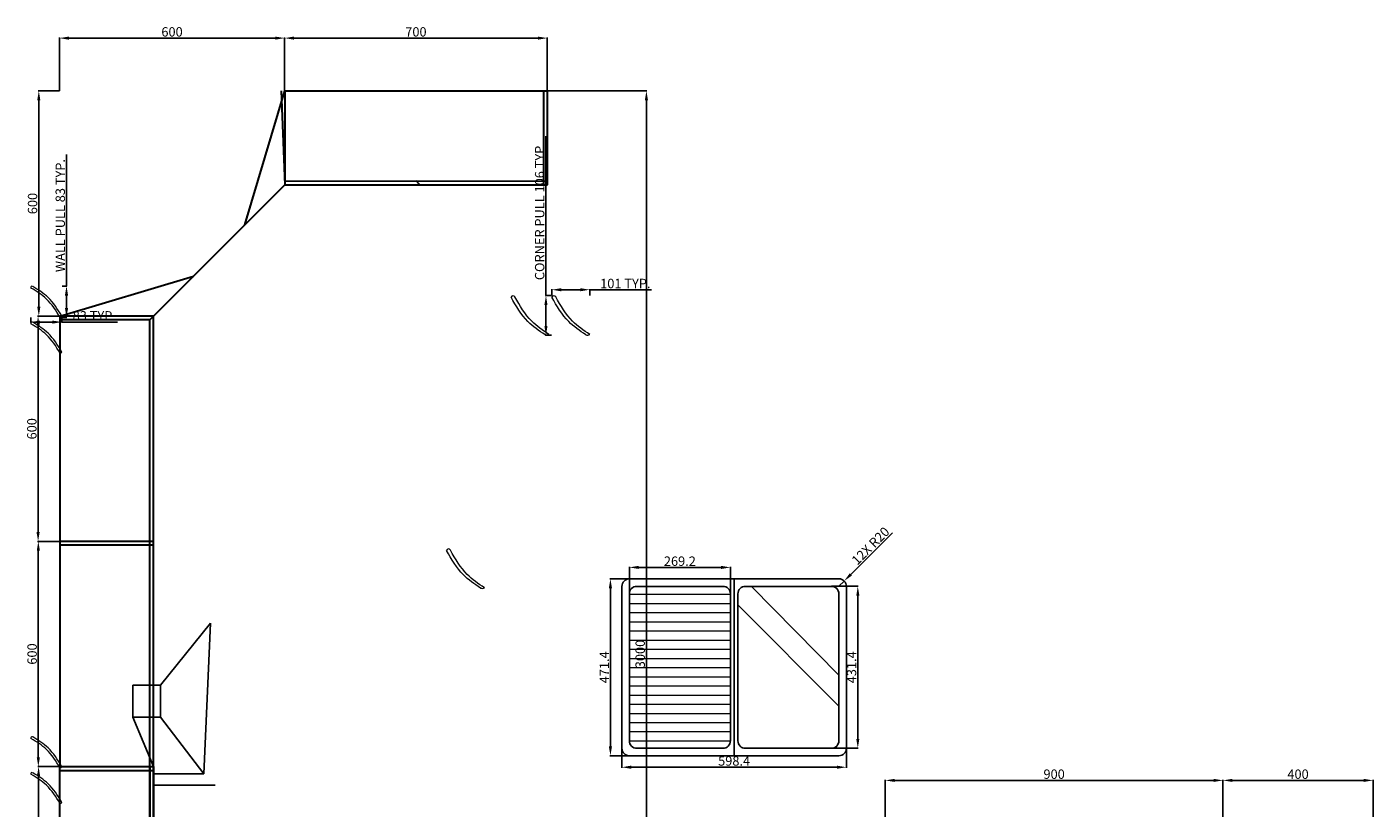
# Model space of a CAD drawing. Units: millimetres. Extents: x 11557 to 15272, y 8572 to 13242.
# Tile 4 of 4: x 11557 to 15145, y 11161 to 13242. Entities that reach past the tile are written whole.
import ezdxf

# ---------------------------------------------------------------- set-up
doc = ezdxf.new("R2010")
doc.units = ezdxf.units.MM
for name, color, linetype, lineweight in [('A-ANNO-DIMS', 2, 'Continuous', 18), ('A-EQPM', 9, 'Continuous', 25), ('A-FIXT-PATT', 8, 'Continuous', 13), ('A-FLOR-FIXT', 4, 'Continuous', 25), ('A-FURN-HARD', 8, 'Continuous', 18), ('A-FURN-WALL', 7, 'Continuous', 30)]:
    doc.layers.add(name, color=color, linetype=linetype, lineweight=lineweight)
doc.styles.get("Standard").update_dxf_attribs({"font": 'arial.ttf'})
doc.dimstyles.new('ISO-25', dxfattribs={"dimtxt": 25, "dimasz": 25, "dimexe": 1.25, "dimexo": 0.625, "dimtad": 1, "dimdec": 1, "dimtxsty": 'Standard', "dimcen": 2.5, "dimadec": 0, "dimazin": 0, "dimtfac": 1, "dimtdec": 1, "dimtmove": 0, "dimatfit": 3, "dimfxl": 1, "dimarcsym": 0})

# ---------------------------------------------------------------- blocks, each defined once
blk = doc.blocks.new('*D5')
at = {"layer": 'A-ANNO-DIMS', "color": 0, "lineweight": -2, "transparency": 16777216}
for p, q in [((13844.6, 11098.9), (13844.6, 11236.3)), ((13869.6, 11235), (14719.6, 11235)), ((14744.6, 11098.9), (14744.6, 11236.3))]:
    blk.add_line(p, q, dxfattribs=at)
at = {"layer": 'A-ANNO-DIMS', "color": 0, "transparency": 16777216}
for points in [[(13869.6, 11239.2), (13869.6, 11230.9), (13844.6, 11235)], [(14719.6, 11239.2), (14719.6, 11230.9), (14744.6, 11235)]]:
    blk.add_solid(points, dxfattribs=at)
at = {"layer": 'Defpoints', "color": 0, "transparency": 16777216}
for p in [(14744.6, 11235), (13844.6, 11098.2, 720), (14744.6, 11098.2, 720)]:
    blk.add_point(p, dxfattribs=at)
at = {"layer": 'A-ANNO-DIMS', "color": 0, "transparency": 16777216, "insert": (14294.6, 11248.4), "char_height": 25, "attachment_point": 5}
blk.add_mtext('900', dxfattribs=at)
blk = doc.blocks.new('*D6')
at = {"layer": 'A-ANNO-DIMS', "color": 0, "lineweight": -2, "transparency": 16777216}
for p, q in [((14744.6, 11111.7), (14744.6, 11236.3)), ((15119.6, 11235), (14769.6, 11235)), ((15144.6, 11111.7), (15144.6, 11236.3))]:
    blk.add_line(p, q, dxfattribs=at)
at = {"layer": 'A-ANNO-DIMS', "color": 0, "transparency": 16777216}
for points in [[(14769.6, 11239.2), (14769.6, 11230.9), (14744.6, 11235)], [(15119.6, 11239.2), (15119.6, 11230.9), (15144.6, 11235)]]:
    blk.add_solid(points, dxfattribs=at)
at = {"layer": 'Defpoints', "color": 0, "transparency": 16777216}
for p in [(14744.6, 11235), (14744.6, 11111, 720), (15144.6, 11111, 720)]:
    blk.add_point(p, dxfattribs=at)
at = {"layer": 'A-ANNO-DIMS', "color": 0, "transparency": 16777216, "insert": (14944.6, 11248.4), "char_height": 25, "attachment_point": 5}
blk.add_mtext('400', dxfattribs=at)
blk = doc.blocks.new('*D8')
at = {"layer": 'A-ANNO-DIMS', "color": 0, "lineweight": -2, "transparency": 16777216}
for p, q in [((11643.1, 11271.7), (11586.9, 11271.7)), ((11588.2, 11246.7), (11588.2, 10696.7)), ((11643.1, 10671.7), (11586.9, 10671.7))]:
    blk.add_line(p, q, dxfattribs=at)
at = {"layer": 'A-ANNO-DIMS', "color": 0, "transparency": 16777216}
for points in [[(11584, 11246.7), (11592.3, 11246.7), (11588.2, 11271.7)], [(11584, 10696.7), (11592.3, 10696.7), (11588.2, 10671.7)]]:
    blk.add_solid(points, dxfattribs=at)
at = {"layer": 'Defpoints', "color": 0, "transparency": 16777216}
for p in [(11643.8, 11271.7, 720), (11588.2, 10671.7), (11643.8, 10671.7, 720)]:
    blk.add_point(p, dxfattribs=at)
at = {"layer": 'A-ANNO-DIMS', "color": 0, "transparency": 16777216, "insert": (11574.8, 10971.7), "char_height": 25, "attachment_point": 5, "rotation": 90}
blk.add_mtext('600', dxfattribs=at)
blk = doc.blocks.new('*D9')
at = {"layer": 'A-ANNO-DIMS', "color": 0, "lineweight": -2, "transparency": 16777216}
for p, q in [((11642.5, 11871.7), (11586.3, 11871.7)), ((11587.5, 11846.7), (11587.5, 11296.7)), ((11642.5, 11271.7), (11586.3, 11271.7))]:
    blk.add_line(p, q, dxfattribs=at)
at = {"layer": 'A-ANNO-DIMS', "color": 0, "transparency": 16777216}
for points in [[(11583.4, 11846.7), (11591.7, 11846.7), (11587.5, 11871.7)], [(11583.4, 11296.7), (11591.7, 11296.7), (11587.5, 11271.7)]]:
    blk.add_solid(points, dxfattribs=at)
at = {"layer": 'Defpoints', "color": 0, "transparency": 16777216}
for p in [(11643.1, 11871.7, 720), (11587.5, 11271.7), (11643.1, 11271.7, 720)]:
    blk.add_point(p, dxfattribs=at)
at = {"layer": 'A-ANNO-DIMS', "color": 0, "transparency": 16777216, "insert": (11574.1, 11571.7), "char_height": 25, "attachment_point": 5, "rotation": 90}
blk.add_mtext('600', dxfattribs=at)
blk = doc.blocks.new('*D10')
at = {"layer": 'A-ANNO-DIMS', "color": 0, "lineweight": -2, "transparency": 16777216}
for p, q in [((11641.9, 12471.7), (11585.7, 12471.7)), ((11586.9, 12446.7), (11586.9, 11896.7)), ((11641.9, 11871.7), (11585.7, 11871.7))]:
    blk.add_line(p, q, dxfattribs=at)
at = {"layer": 'A-ANNO-DIMS', "color": 0, "transparency": 16777216}
for points in [[(11582.7, 12446.7), (11591.1, 12446.7), (11586.9, 12471.7)], [(11582.7, 11896.7), (11591.1, 11896.7), (11586.9, 11871.7)]]:
    blk.add_solid(points, dxfattribs=at)
at = {"layer": 'Defpoints', "color": 0, "transparency": 16777216}
for p in [(11642.5, 12471.7, 720), (11586.9, 11871.7), (11642.5, 11871.7, 720)]:
    blk.add_point(p, dxfattribs=at)
at = {"layer": 'A-ANNO-DIMS', "color": 0, "transparency": 16777216, "insert": (11573.5, 12171.7), "char_height": 25, "attachment_point": 5, "rotation": 90}
blk.add_mtext('600', dxfattribs=at)
blk = doc.blocks.new('*D11')
at = {"layer": 'A-ANNO-DIMS', "color": 0, "lineweight": -2, "transparency": 16777216}
for p, q in [((11643.8, 13071.7), (11587.5, 13071.7)), ((11588.8, 13046.7), (11588.8, 12496.7)), ((11643.8, 12471.7), (11587.5, 12471.7))]:
    blk.add_line(p, q, dxfattribs=at)
at = {"layer": 'A-ANNO-DIMS', "color": 0, "transparency": 16777216}
for points in [[(11584.6, 13046.7), (11592.9, 13046.7), (11588.8, 13071.7)], [(11584.6, 12496.7), (11592.9, 12496.7), (11588.8, 12471.7)]]:
    blk.add_solid(points, dxfattribs=at)
at = {"layer": 'Defpoints', "color": 0, "transparency": 16777216}
for p in [(11644.4, 13071.7, 720), (11588.8, 12471.7), (11644.4, 12471.7, 720)]:
    blk.add_point(p, dxfattribs=at)
at = {"layer": 'A-ANNO-DIMS', "color": 0, "transparency": 16777216, "insert": (11575.4, 12771.7), "char_height": 25, "attachment_point": 5, "rotation": 90}
blk.add_mtext('600', dxfattribs=at)
blk = doc.blocks.new('*D12')
at = {"layer": 'A-ANNO-DIMS', "color": 0, "lineweight": -2, "transparency": 16777216}
for p, q in [((11643.8, 13071.7), (11643.8, 13213.6)), ((11668.8, 13212.4), (12218.8, 13212.4)), ((12243.8, 13071.7), (12243.8, 13213.6))]:
    blk.add_line(p, q, dxfattribs=at)
at = {"layer": 'A-ANNO-DIMS', "color": 0, "transparency": 16777216}
for points in [[(11668.8, 13216.5), (11668.8, 13208.2), (11643.8, 13212.4)], [(12218.8, 13216.5), (12218.8, 13208.2), (12243.8, 13212.4)]]:
    blk.add_solid(points, dxfattribs=at)
at = {"layer": 'Defpoints', "color": 0, "transparency": 16777216}
for p in [(12243.8, 13212.4), (11643.8, 13071, 250), (12243.8, 13071, 250)]:
    blk.add_point(p, dxfattribs=at)
at = {"layer": 'A-ANNO-DIMS', "color": 0, "transparency": 16777216, "insert": (11943.8, 13225.8), "char_height": 25, "attachment_point": 5}
blk.add_mtext('600', dxfattribs=at)
blk = doc.blocks.new('*D13')
at = {"layer": 'A-ANNO-DIMS', "color": 0, "lineweight": -2, "transparency": 16777216}
for p, q in [((12243.8, 13071.7), (12243.8, 13213.6)), ((12268.8, 13212.4), (12918.8, 13212.4)), ((12943.8, 13071.7), (12943.8, 13213.6))]:
    blk.add_line(p, q, dxfattribs=at)
at = {"layer": 'A-ANNO-DIMS', "color": 0, "transparency": 16777216}
for points in [[(12268.8, 13216.5), (12268.8, 13208.2), (12243.8, 13212.4)], [(12918.8, 13216.5), (12918.8, 13208.2), (12943.8, 13212.4)]]:
    blk.add_solid(points, dxfattribs=at)
at = {"layer": 'Defpoints', "color": 0, "transparency": 16777216}
for p in [(12943.8, 13212.4), (12243.8, 13071, 250), (12943.8, 13071, 250)]:
    blk.add_point(p, dxfattribs=at)
at = {"layer": 'A-ANNO-DIMS', "color": 0, "transparency": 16777216, "insert": (12593.8, 13225.8), "char_height": 25, "attachment_point": 5}
blk.add_mtext('700', dxfattribs=at)
blk = doc.blocks.new('WALL-CABINET-PULL')
for centre, radius, start, end in [((3, 79.7, -592.8), 3.04, 50.0455, 215.1607), ((79.2, 3.1, -592.8), 3.13, 238.0113, 27.1949)]:
    blk.add_arc(centre, radius, start, end)
for points in [[(77.6, 0.5, -592.8), (66.9, 17.8, -592.8), (47.2, 49.7, -592.8), (15.2, 69.1, -592.8), (0.5, 77.9, -592.8)], [(82, 4.6, -592.8), (71.3, 21.8, -592.8), (51.6, 53.8, -592.8), (19.6, 73.1, -592.8), (5, 82, -592.8)]]:
    blk.add_open_spline(points, degree=3, knots=[0, 0, 0, 0, 59.935873, 110.632609, 110.632609, 110.632609, 110.632609])
blk = doc.blocks.new('CORNER-CABINET-PULL')
for centre, radius, start, end in [((5.3, 99.5), 5.42, 22.6463, 165.793), ((94.8, 11.5), 11.5, 247.6499, 300.7894)]:
    blk.add_arc(centre, radius, start, end)
for points in [[(90.5, 0.9), (74.3, 11.8), (36.3, 37.7), (13.3, 77.8), (0, 100.8)], [(100.7, 1.6), (84.6, 12.6), (46.6, 38.5), (23.5, 78.5), (10.3, 101.6)]]:
    blk.add_open_spline(points, degree=3, knots=[0, 0, 0, 0, 57.802387, 136.347052, 136.347052, 136.347052, 136.347052])
blk = doc.blocks.new('*D25')
at = {"layer": 'A-ANNO-DIMS', "color": 0, "lineweight": -2, "transparency": 16777216}
for p, q in [((11662.6, 12551.7), (11662.6, 12902.5)), ((11650.7, 12551.7), (11663.9, 12551.7)), ((11662.6, 12493.4), (11662.6, 12526.7)), ((11650.7, 12468.4), (11663.9, 12468.4))]:
    blk.add_line(p, q, dxfattribs=at)
at = {"layer": 'A-ANNO-DIMS', "color": 0, "transparency": 16777216}
for points in [[(11658.4, 12526.7), (11666.8, 12526.7), (11662.6, 12551.7)], [(11658.4, 12493.4), (11666.8, 12493.4), (11662.6, 12468.4)]]:
    blk.add_solid(points, dxfattribs=at)
at = {"layer": 'Defpoints', "color": 0, "transparency": 16777216}
for p in [(11650.1, 12551.7), (11662.6, 12551.7), (11650.1, 12468.4)]:
    blk.add_point(p, dxfattribs=at)
at = {"layer": 'A-ANNO-DIMS', "color": 0, "transparency": 16777216, "insert": (11649.2, 12739.6), "char_height": 25, "attachment_point": 5, "rotation": 90}
blk.add_mtext('WALL PULL 83 TYP.', dxfattribs=at)
blk = doc.blocks.new('*D26')
at = {"layer": 'A-ANNO-DIMS', "color": 0, "lineweight": -2, "transparency": 16777216}
for p, q in [((11567.1, 12467.7), (11567.1, 12454.6)), ((11592.1, 12455.9), (11625.1, 12455.9)), ((11650.1, 12467.7), (11650.1, 12454.6)), ((11650.1, 12455.9), (11798.1, 12455.9))]:
    blk.add_line(p, q, dxfattribs=at)
at = {"layer": 'A-ANNO-DIMS', "color": 0, "transparency": 16777216}
for points in [[(11592.1, 12460), (11592.1, 12451.7), (11567.1, 12455.9)], [(11625.1, 12460), (11625.1, 12451.7), (11650.1, 12455.9)]]:
    blk.add_solid(points, dxfattribs=at)
at = {"layer": 'Defpoints', "color": 0, "transparency": 16777216}
for p in [(11567.1, 12468.4), (11650.1, 12468.4), (11650.1, 12455.9)]:
    blk.add_point(p, dxfattribs=at)
at = {"layer": 'A-ANNO-DIMS', "color": 0, "transparency": 16777216, "insert": (11736.6, 12469.3), "char_height": 25, "attachment_point": 5}
blk.add_mtext('83 TYP.', dxfattribs=at)
blk = doc.blocks.new('*D27')
at = {"layer": 'A-ANNO-DIMS', "color": 0, "lineweight": -2, "transparency": 16777216}
for p, q in [((12940.3, 12526.3), (12940.3, 12951.5)), ((12955.5, 12526.3), (12939.1, 12526.3)), ((12940.3, 12445.7), (12940.3, 12501.3)), ((12955.5, 12420.7), (12939.1, 12420.7))]:
    blk.add_line(p, q, dxfattribs=at)
at = {"layer": 'A-ANNO-DIMS', "color": 0, "transparency": 16777216}
for points in [[(12936.2, 12501.3), (12944.5, 12501.3), (12940.3, 12526.3)], [(12936.2, 12445.7), (12944.5, 12445.7), (12940.3, 12420.7)]]:
    blk.add_solid(points, dxfattribs=at)
at = {"layer": 'Defpoints', "color": 0, "transparency": 16777216}
for p in [(12940.3, 12526.3), (12956.2, 12526.3), (12956.2, 12420.7)]:
    blk.add_point(p, dxfattribs=at)
at = {"layer": 'A-ANNO-DIMS', "color": 0, "transparency": 16777216, "insert": (12926.8, 12751.4), "char_height": 25, "attachment_point": 5, "rotation": 90}
blk.add_mtext('CORNER PULL 106 TYP.', dxfattribs=at)
blk = doc.blocks.new('*D28')
at = {"layer": 'A-ANNO-DIMS', "color": 0, "lineweight": -2, "transparency": 16777216}
for p, q in [((12956.2, 12526.9), (12956.2, 12543.4)), ((12981.2, 12542.1), (13031.9, 12542.1)), ((13056.9, 12526.9), (13056.9, 12543.4)), ((13056.9, 12542.1), (13221.9, 12542.1))]:
    blk.add_line(p, q, dxfattribs=at)
at = {"layer": 'A-ANNO-DIMS', "color": 0, "transparency": 16777216}
for points in [[(12981.2, 12546.3), (12981.2, 12537.9), (12956.2, 12542.1)], [(13031.9, 12546.3), (13031.9, 12537.9), (13056.9, 12542.1)]]:
    blk.add_solid(points, dxfattribs=at)
at = {"layer": 'Defpoints', "color": 0, "transparency": 16777216}
for p in [(12956.2, 12526.3), (13056.9, 12542.1), (13056.9, 12526.3)]:
    blk.add_point(p, dxfattribs=at)
at = {"layer": 'A-ANNO-DIMS', "color": 0, "transparency": 16777216, "insert": (13151.9, 12555.5), "char_height": 25, "attachment_point": 5}
blk.add_mtext('101 TYP.', dxfattribs=at)
blk = doc.blocks.new('*D36')
at = {"layer": 'A-ANNO-DIMS', "color": 0, "lineweight": -2, "transparency": 16777216}
for p, q in [((12944.4, 13071.7), (13209.3, 13071.7)), ((13208.1, 10096.7), (13208.1, 13046.7)), ((11895, 10071.7), (13209.3, 10071.7))]:
    blk.add_line(p, q, dxfattribs=at)
at = {"layer": 'A-ANNO-DIMS', "color": 0, "transparency": 16777216}
for points in [[(13203.9, 13046.7), (13212.2, 13046.7), (13208.1, 13071.7)], [(13203.9, 10096.7), (13212.2, 10096.7), (13208.1, 10071.7)]]:
    blk.add_solid(points, dxfattribs=at)
at = {"layer": 'Defpoints', "color": 0, "transparency": 16777216}
for p in [(12943.8, 13071.7), (13208.1, 13071.7), (11894.4, 10071.7)]:
    blk.add_point(p, dxfattribs=at)
at = {"layer": 'A-ANNO-DIMS', "color": 0, "transparency": 16777216, "insert": (13194.7, 11571.7), "char_height": 25, "attachment_point": 5, "rotation": 90}
blk.add_mtext('3000', dxfattribs=at)
blk = doc.blocks.new('*D37')
at = {"layer": 'A-ANNO-DIMS', "color": 0, "lineweight": -2, "transparency": 16777216}
for p, q in [((13142.6, 11319.9), (13142.6, 11268.8)), ((13741, 11319.9), (13741, 11268.8)), ((13167.6, 11270.1), (13716, 11270.1))]:
    blk.add_line(p, q, dxfattribs=at)
at = {"layer": 'A-ANNO-DIMS', "color": 0, "transparency": 16777216}
for points in [[(13167.6, 11274.3), (13167.6, 11265.9), (13142.6, 11270.1)], [(13716, 11274.3), (13716, 11265.9), (13741, 11270.1)]]:
    blk.add_solid(points, dxfattribs=at)
at = {"layer": 'Defpoints', "color": 0, "transparency": 16777216}
for p in [(13142.6, 11320.5), (13741, 11320.5), (13741, 11270.1)]:
    blk.add_point(p, dxfattribs=at)
at = {"layer": 'A-ANNO-DIMS', "color": 0, "transparency": 16777216, "insert": (13441.8, 11283.5), "char_height": 25, "attachment_point": 5}
blk.add_mtext('598.4', dxfattribs=at)
blk = doc.blocks.new('*D38')
at = {"layer": 'A-ANNO-DIMS', "color": 0, "lineweight": -2, "transparency": 16777216}
for p, q in [((13162, 11772), (13110.9, 11772)), ((13112.2, 11325.5), (13112.2, 11747)), ((13162, 11300.5), (13110.9, 11300.5))]:
    blk.add_line(p, q, dxfattribs=at)
at = {"layer": 'A-ANNO-DIMS', "color": 0, "transparency": 16777216}
for points in [[(13108, 11747), (13116.3, 11747), (13112.2, 11772)], [(13108, 11325.5), (13116.3, 11325.5), (13112.2, 11300.5)]]:
    blk.add_solid(points, dxfattribs=at)
at = {"layer": 'Defpoints', "color": 0, "transparency": 16777216}
for p in [(13112.2, 11772), (13162.6, 11772), (13162.6, 11300.5)]:
    blk.add_point(p, dxfattribs=at)
at = {"layer": 'A-ANNO-DIMS', "color": 0, "transparency": 16777216, "insert": (13099, 11536.3), "char_height": 25, "attachment_point": 5, "rotation": 90}
blk.add_mtext('471.4', dxfattribs=at)
blk = doc.blocks.new('*D39')
at = {"layer": 'A-ANNO-DIMS', "color": 0, "lineweight": -2, "transparency": 16777216}
for p, q in [((13162.6, 11732.6), (13162.6, 11803.7)), ((13431.8, 11732.6), (13431.8, 11803.7)), ((13187.6, 11802.4), (13406.8, 11802.4))]:
    blk.add_line(p, q, dxfattribs=at)
at = {"layer": 'A-ANNO-DIMS', "color": 0, "transparency": 16777216}
for points in [[(13187.6, 11806.6), (13187.6, 11798.2), (13162.6, 11802.4)], [(13406.8, 11806.6), (13406.8, 11798.2), (13431.8, 11802.4)]]:
    blk.add_solid(points, dxfattribs=at)
at = {"layer": 'Defpoints', "color": 0, "transparency": 16777216}
for p in [(13431.8, 11802.4), (13162.6, 11732), (13431.8, 11732)]:
    blk.add_point(p, dxfattribs=at)
at = {"layer": 'A-ANNO-DIMS', "color": 0, "transparency": 16777216, "insert": (13297.2, 11815.8), "char_height": 25, "attachment_point": 5}
blk.add_mtext('269.2', dxfattribs=at)
blk = doc.blocks.new('*D40')
at = {"layer": 'A-ANNO-DIMS', "color": 0, "lineweight": -2, "transparency": 16777216}
for p, q in [((13701.6, 11752), (13772.7, 11752)), ((13771.4, 11345.5), (13771.4, 11727)), ((13701.6, 11320.5), (13772.7, 11320.5))]:
    blk.add_line(p, q, dxfattribs=at)
at = {"layer": 'A-ANNO-DIMS', "color": 0, "transparency": 16777216}
for points in [[(13767.3, 11727), (13775.6, 11727), (13771.4, 11752)], [(13767.3, 11345.5), (13775.6, 11345.5), (13771.4, 11320.5)]]:
    blk.add_solid(points, dxfattribs=at)
at = {"layer": 'Defpoints', "color": 0, "transparency": 16777216}
for p in [(13701, 11752), (13771.4, 11752), (13701, 11320.5)]:
    blk.add_point(p, dxfattribs=at)
at = {"layer": 'A-ANNO-DIMS', "color": 0, "transparency": 16777216, "insert": (13758, 11536.3), "char_height": 25, "attachment_point": 5, "rotation": 90}
blk.add_mtext('431.4', dxfattribs=at)
blk = doc.blocks.new('*D49')
at = {"layer": 'A-ANNO-DIMS', "color": 0, "lineweight": -2, "transparency": 16777216}
for p, q in [((13863.6, 11894.6), (13752.8, 11783.8)), ((13721, 11752), (13735.1, 11766.1))]:
    blk.add_line(p, q, dxfattribs=at)
at = {"layer": 'A-ANNO-DIMS', "color": 0, "transparency": 16777216}
blk.add_solid([(13749.9, 11786.7), (13755.7, 11780.8), (13735.1, 11766.1)], dxfattribs=at)
at = {"layer": 'Defpoints', "color": 0, "transparency": 16777216}
for p in [(13721, 11752), (13735.1, 11766.1)]:
    blk.add_point(p, dxfattribs=at)
at = {"layer": 'A-ANNO-DIMS', "color": 0, "transparency": 16777216, "insert": (13807.6, 11857.5), "char_height": 25, "attachment_point": 5, "rotation": 45.0126}
blk.add_mtext('12X R20', dxfattribs=at)

msp = doc.modelspace()

# ---------------------------------------------------------------- hatches: boundary and pattern name
at = {"layer": 'A-FIXT-PATT'}
h = msp.add_hatch(dxfattribs=at)
h.set_pattern_fill('ANSI31', color=256, scale=7.6813, angle=135, style=0)
h.paths.add_polyline_path([(13411.798, 11320.545), (13415.271, 11320.849), (13418.638, 11321.751), (13421.798, 11323.224), (13424.654, 11325.224), (13427.119, 11327.689), (13429.118, 11330.545), (13430.592, 11333.704), (13431.494, 11337.072), (13431.798, 11340.545), (13431.798, 11731.963), (13431.494, 11735.436), (13430.592, 11738.803), (13429.118, 11741.963), (13427.119, 11744.819), (13424.654, 11747.284), (13421.798, 11749.283), (13418.638, 11750.757), (13415.271, 11751.659), (13411.798, 11751.963), (13182.607, 11751.963), (13179.134, 11751.659), (13175.766, 11750.757), (13172.607, 11749.283), (13169.751, 11747.284), (13167.286, 11744.819), (13165.286, 11741.963), (13163.813, 11738.803), (13162.911, 11735.436), (13162.607, 11731.963), (13162.607, 11340.545), (13162.911, 11337.072), (13163.813, 11333.704), (13165.286, 11330.545), (13167.286, 11327.689), (13169.751, 11325.224), (13172.607, 11323.224), (13175.766, 11321.751), (13179.134, 11320.849), (13182.607, 11320.545)])

# ---------------------------------------------------------------- linework, layer by layer
at = {"layer": 'A-EQPM'}
for p, q in [((11912.959, 11488.658, -261.749), (12046.196, 11653.568, -452.435)), ((12028.469, 11252.251, -470), (12046.196, 11653.568, -452.435)), ((12028.469, 11252.251, -500), (12046.196, 11653.568, -482.273)), ((12046.196, 11653.568, -452.435), (12046.196, 11653.568, -482.273)), ((11912.959, 11488.658), (11912.959, 11488.658, -252.638)), ((11912.959, 11488.658, -252.638), (11912.959, 11488.658, -261.749)), ((11912.959, 11403.186, -261.749), (11912.959, 11488.658, -261.749)), ((11839.699, 11403.186), (11839.699, 11403.186, -261.749)), ((11912.959, 11403.186, -261.749), (11839.699, 11403.186, -261.749)), ((11839.699, 11403.186, -261.749), (11894.396, 11271.656, -231.822)), ((11912.959, 11403.186), (11912.959, 11403.186, -261.749)), ((11912.959, 11403.186, -261.749), (12028.469, 11252.251, -470)), ((11894.396, 11252.251, -470), (12028.469, 11252.251, -470)), ((12028.469, 11252.251, -470), (12028.469, 11252.251, -500)), ((11894.396, 11222.251, -470), (12058.469, 11222.251, -470))]:
    msp.add_line(p, q, dxfattribs=at)
msp.add_lwpolyline([(11839.699, 11403.186), (11912.959, 11403.186), (11912.959, 11488.658), (11839.699, 11488.658)], close=True, dxfattribs=at)
at = {"layer": 'A-FLOR-FIXT'}
for p, q in [((13441.798, 11300.545), (13441.798, 11771.963)), ((13411.798, 11751.963), (13379.785, 11751.963)), ((13431.798, 11340.545), (13431.798, 11731.963)), ((13451.798, 11340.545), (13451.798, 11731.963)), ((13471.798, 11751.963), (13503.811, 11751.963)), ((13487.804, 11751.963), (13720.989, 11515.061)), ((13451.798, 11702.42), (13720.989, 11432.637)), ((13411.798, 11320.545), (13381.333, 11320.545))]:
    msp.add_line(p, q, dxfattribs=at)
msp.add_lwpolyline([(13162.607, 11300.545), (13720.989, 11300.545, 0.41421356), (13740.989, 11320.545), (13740.989, 11751.963, 0.41421356), (13720.989, 11771.963), (13162.607, 11771.963, 0.41421356), (13142.607, 11751.963), (13142.607, 11320.545, 0.41421356)], format="xyb", close=True, dxfattribs=at)
for points in [[(13411.798, 11751.963), (13182.607, 11751.963, 0.41421356), (13162.607, 11731.963), (13162.607, 11340.545, 0.41421356), (13182.607, 11320.545), (13411.798, 11320.545)], [(13471.798, 11751.963), (13700.989, 11751.963, -0.41421356), (13720.989, 11731.963), (13720.989, 11340.545, -0.41421356), (13700.989, 11320.545), (13471.798, 11320.545)]]:
    msp.add_lwpolyline(points, format="xyb", dxfattribs=at)
for centre, start, end in [((13411.798, 11731.963), 0, 90), ((13471.798, 11731.963), 90, 180), ((13411.798, 11340.545), 270, 0), ((13471.798, 11340.545), 180, 270)]:
    msp.add_arc(centre, 20, start, end, dxfattribs=at)
at = {"layer": 'A-FURN-HARD'}
for centre, radius, start, end in [((12680.692, 11846.03, 385.918), 5.418, 22.646306, 165.792972), ((12770.269, 11758.02, 385.918), 11.492, 247.649873, 300.789404)]:
    msp.add_arc(centre, radius, start, end, dxfattribs=at)
for points in [[(12765.9, 11747.392, 385.918), (12749.789, 11758.364, 385.918), (12711.786, 11784.244, 385.918), (12688.725, 11824.29, 385.918), (12675.44, 11847.359, 385.918)], [(12776.152, 11748.149, 385.918), (12760.041, 11759.12, 385.918), (12722.038, 11785, 385.918), (12698.977, 11825.047, 385.918), (12685.692, 11848.116, 385.918)]]:
    msp.add_open_spline(points, degree=3, knots=[0, 0, 0, 0, 57.80238671, 136.34705222, 136.34705222, 136.34705222, 136.34705222], dxfattribs=at)
at = {"layer": 'A-FURN-WALL'}
for p, q in [((12137.399, 12714.659, 606.997), (12244.396, 13071.656, 250)), ((12234.396, 13071.656, 250), (12244.396, 12821.656, 260)), ((12243.771, 13071.656, 250), (12943.771, 13071.656, 250)), ((12244.396, 13071.656, 250), (12244.396, 12821.656, 250)), ((12933.771, 13071.656, 250), (12933.771, 12822.281, 250)), ((12943.771, 13071.656, 250), (12943.771, 12822.281, 250)), ((12943.771, 13071.656, 250), (12943.771, 13071.656, -470)), ((12943.771, 13071.656, -470), (12943.771, 12821.656, -470)), ((12244.396, 12821.656, 260), (11884.396, 12461.656, 260)), ((12244.396, 12821.656, 250), (11894.396, 12471.656, 250)), ((11894.396, 12471.656, -470), (12244.396, 12821.656, -470)), ((12244.396, 12831.656, 250), (12943.77, 12832.282, 250.607)), ((12244.396, 12821.656, 250), (12943.77, 12822.282, 250.607)), ((12244.396, 12821.656, 250), (12244.396, 12821.656, -470)), ((12244.396, 12821.656, -470), (12944.396, 12821.656, -470)), ((12604.074, 12821.978, 250.312), (12594.083, 12831.969, -480.313)), ((12934.396, 12821.656, -470), (12933.771, 12822.281, 250)), ((12944.396, 12821.656, -470), (12943.771, 12822.281, 250)), ((12137.399, 12714.659, 606.997), (12001.393, 12578.654, 606.997)), ((11644.396, 12471.656, 250), (12001.393, 12578.654, 606.997)), ((11894.396, 12471.656, 250), (11644.396, 12471.656, 250)), ((11644.396, 12471.656, 250), (11644.396, 11871.656, 250)), ((11884.396, 12461.656, 250), (11644.396, 12461.656, 250)), ((11884.396, 11871.656, 250), (11884.396, 12461.656, 250)), ((11894.396, 11871.656, 250), (11894.396, 12471.656, 250)), ((11894.396, 11871.656, -470), (11894.396, 12471.656, -470)), ((11894.396, 12471.656, -470), (11894.396, 12471.656, 250)), ((11894.396, 12171.656, 250), (11894.396, 12171.656, -470)), ((11894.396, 11871.656, 250), (11644.396, 11871.656, 250)), ((11644.396, 11871.656, 250), (11644.396, 11271.656, 250)), ((11894.396, 11871.656, -470), (11644.396, 11871.656, -470)), ((11644.396, 11871.656, -470), (11644.396, 11871.656)), ((11894.396, 11861.656, 250), (11644.396, 11861.656, 250)), ((11884.396, 11271.656, 250), (11884.396, 11871.656, 250)), ((11884.396, 11271.656, 250), (11884.396, 11871.656, 250)), ((11894.396, 11271.656, 250), (11894.396, 11871.656, 250)), ((11894.396, 11871.656, -470), (11894.396, 11871.656, 250)), ((11894.396, 11271.656, 250), (11894.396, 11871.656, 250)), ((11644.396, 10671.656, 250), (11644.396, 11271.656, 250)), ((11644.396, 11271.656, 250), (11894.396, 11271.656, 250)), ((11884.396, 11271.656, 250), (11884.396, 10671.656, 250)), ((11884.396, 10671.656, 250), (11884.396, 11271.656, 250)), ((11894.396, 11271.656, 250), (11894.396, 10671.656, 250)), ((11894.396, 10671.656, 250), (11894.396, 11271.656, 250)), ((11894.396, 10671.656, -470), (11894.396, 11271.656, -470)), ((11894.396, 11271.656, -470), (11894.396, 11271.656, 250)), ((11644.396, 11261.656, 250), (11894.396, 11261.656, 250))]:
    msp.add_line(p, q, dxfattribs=at)

# ---------------------------------------------------------------- block references
at = {"layer": 'A-FURN-HARD'}
for name, p in [('WALL-CABINET-PULL', (11567.456, 12468.644)), ('CORNER-CABINET-PULL', (12847.433, 12421.197)), ('CORNER-CABINET-PULL', (12956.164, 12421.197)), ('WALL-CABINET-PULL', (11567.456, 12373.337)), ('WALL-CABINET-PULL', (11567.456, 11268.644)), ('WALL-CABINET-PULL', (11567.456, 11173.337))]:
    msp.add_blockref(name, p, dxfattribs=at)

# ---------------------------------------------------------------- dimensions: what is measured, and where the dimension line sits
at = {"layer": 'A-ANNO-DIMS'}
for base, p1, p2, picture, middle in [((12243.771, 13212.375, 250), (11643.771, 13071.031, 500), (12243.771, 13071.031, 500), '*D12', (11943.771, 13212.375, 250)), ((14744.618, 11235.018, 720), (13844.618, 11098.234, 1440), (14744.618, 11098.234, 1440), '*D5', (14294.618, 11235.018, 720))]:
    dim = msp.add_linear_dim(base=base, p1=p1, p2=p2, dimstyle='ISO-25', override={"dimclrd": 0, "dimclre": 0, "dimclrt": 0}, dxfattribs=at)
    dim.commit()
    dim.dimension.update_dxf_attribs({"geometry": picture, "text_midpoint": middle, "dimtype": 160})
for base, p1, p2, override, picture, middle in [((12943.771, 13212.375, 250), (12243.771, 13071.031, 500), (12943.771, 13071.031, 500), {"dimclrd": 0, "dimclre": 0, "dimclrt": 0}, '*D13', (12593.771, 13225.764, 250)), ((13431.798, 11802.413), (13162.607, 11731.963), (13431.798, 11731.963), {"dimdec": 1, "dimlfac": 1, "dimrnd": 0, "dimzin": 0, "dimdsep": 46, "dimlunit": 2}, '*D39', (13297.202, 11815.802)), ((13740.989, 11270.095), (13142.607, 11320.545), (13740.989, 11320.545), {"dimdec": 1, "dimlfac": 1, "dimrnd": 0, "dimzin": 0, "dimdsep": 46, "dimlunit": 2}, '*D37', (13441.798, 11283.484)), ((14744.618, 11235.018, 720), (15144.618, 11111.04, 1440), (14744.618, 11111.04, 1440), {"dimclrd": 0, "dimclre": 0, "dimclrt": 0}, '*D6', (14944.618, 11248.408, 720))]:
    dim = msp.add_linear_dim(base=base, p1=p1, p2=p2, dimstyle='ISO-25', override=override, dxfattribs=at)
    dim.commit()
    dim.dimension.update_dxf_attribs({"geometry": picture, "text_midpoint": middle})
for base, p1, p2, picture, middle in [((11588.776, 12471.656, 250), (11644.396, 13071.656, 970), (11644.396, 12471.656, 970), '*D11', (11588.776, 12771.656, 250)), ((11586.901, 11871.656, 250), (11642.521, 12471.656, 970), (11642.521, 11871.656, 970), '*D10', (11586.901, 12171.656, 250)), ((11587.526, 11271.656, 250), (11643.146, 11871.656, 970), (11643.146, 11271.656, 970), '*D9', (11587.526, 11571.656, 250)), ((11588.151, 10671.656, 250), (11643.771, 11271.656, 970), (11643.771, 10671.656, 970), '*D8', (11588.151, 10971.656, 250))]:
    dim = msp.add_linear_dim(base=base, p1=p1, p2=p2, angle=90, dimstyle='ISO-25', override={"dimclrd": 0, "dimclre": 0, "dimclrt": 0}, dxfattribs=at)
    dim.commit()
    dim.dimension.update_dxf_attribs({"geometry": picture, "text_midpoint": middle, "dimtype": 160})
for base, p1, p2, override, picture, middle in [((13208.076, 13071.656), (11894.396, 10071.656), (12943.771, 13071.656), {"dimdec": 0, "dimlfac": 1, "dimrnd": 0, "dimzin": 0, "dimdsep": 46, "dimlunit": 2}, '*D36', (13194.678, 11571.656)), ((13112.157, 11771.963), (13162.607, 11300.545), (13162.607, 11771.963), {"dimdec": 1, "dimlfac": 1, "dimrnd": 0, "dimzin": 0, "dimdsep": 46, "dimlunit": 2}, '*D38', (13098.981, 11536.254)), ((13771.439, 11751.963), (13700.989, 11320.545), (13700.989, 11751.963), {"dimdec": 1, "dimlfac": 1, "dimrnd": 0, "dimzin": 0, "dimdsep": 46, "dimlunit": 2}, '*D40', (13758.041, 11536.254))]:
    dim = msp.add_linear_dim(base=base, p1=p1, p2=p2, angle=90, dimstyle='ISO-25', override=override, dxfattribs=at)
    dim.commit()
    dim.dimension.update_dxf_attribs({"geometry": picture, "text_midpoint": middle})
for base, p1, p2, text, picture, middle in [((12940.326, 12526.262), (12956.164, 12420.674), (12956.164, 12526.262), 'CORNER PULL <> TYP.', '*D27', (12926.766, 12751.359)), ((11662.604, 12551.662), (11650.11, 12468.366), (11650.11, 12551.662), 'WALL PULL <> TYP.', '*D25', (11649.206, 12739.583))]:
    dim = msp.add_linear_dim(base=base, p1=p1, p2=p2, angle=90, text=text, dimstyle='ISO-25', override={"dimdec": 0, "dimlfac": 1, "dimrnd": 0, "dimzin": 0, "dimdsep": 46, "dimlunit": 2}, dxfattribs=at)
    dim.commit()
    dim.dimension.update_dxf_attribs({"geometry": picture, "text_midpoint": middle})
for base, p1, p2, picture, middle in [((13056.876, 12542.101), (12956.164, 12526.262), (13056.876, 12526.262), '*D28', (13151.882, 12555.49)), ((11650.11, 12455.871), (11567.124, 12468.366), (11650.11, 12468.366), '*D26', (11736.598, 12469.269))]:
    dim = msp.add_linear_dim(base=base, p1=p1, p2=p2, text='<> TYP.', dimstyle='ISO-25', override={"dimdec": 0, "dimlfac": 1, "dimrnd": 0, "dimzin": 0, "dimdsep": 46, "dimlunit": 2}, dxfattribs=at)
    dim.commit()
    dim.dimension.update_dxf_attribs({"geometry": picture, "text_midpoint": middle})
dim = msp.add_radius_dim(center=(13720.989, 11751.963), mpoint=(13735.128, 11766.108), text='12X <>', dimstyle='ISO-25', override={"dimdec": 0, "dimlfac": 1, "dimrnd": 0, "dimzin": 0, "dimdsep": 46, "dimlunit": 2}, dxfattribs=at)
dim.commit()
dim.dimension.update_dxf_attribs({"geometry": '*D49', "text_midpoint": (13807.555, 11857.507)})

doc.saveas('drawing.dxf')
